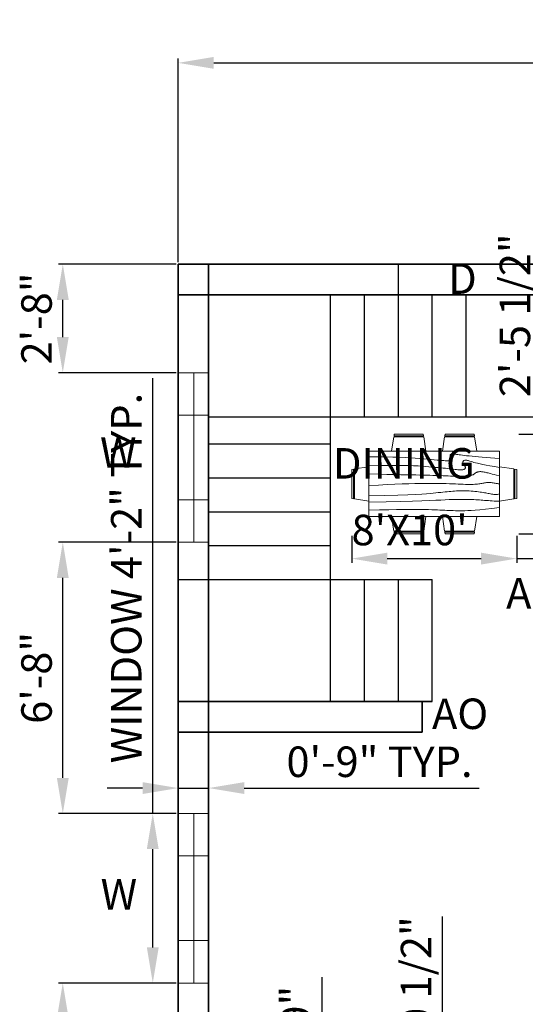
# Model space of a CAD drawing. Units: inches. Extents: x 1956 to 4770, y 1551 to 2596.
# Tile 6 of 10: x 2211 to 2361, y 2091 to 2381. Entities that reach past the tile are written whole.
import ezdxf

# ---------------------------------------------------------------- set-up
doc = ezdxf.new("R2010")
doc.units = ezdxf.units.IN
for name, color, linetype, lineweight in [('A-ANNO-DIMS', 2, 'Continuous', 18), ('A-ANNO-TEXT', 7, 'Continuous', 18), ('A-AREA-IDEN', 7, 'Continuous', 18), ('A-FLOR-STRS', 7, 'Continuous', 25), ('A-FURN', 8, 'Continuous', 18), ('A-GLAZ', 4, 'Continuous', 18), ('A-WALL', 7, 'Continuous', 35)]:
    doc.layers.add(name, color=color, linetype=linetype, lineweight=lineweight)
doc.styles.get("Standard").update_dxf_attribs({"font": 'arial.ttf'})
doc.dimstyles.new('ISO-25', dxfattribs={"dimtxt": 9, "dimasz": 10.5, "dimexe": 1.25, "dimexo": 0.625, "dimgap": 2, "dimtad": 1, "dimdec": 1, "dimlunit": 4, "dimtxsty": 'Standard', "dimcen": 2.5, "dimadec": 0, "dimazin": 0, "dimtfac": 1, "dimtdec": 1, "dimtmove": 0, "dimatfit": 3, "dimfxl": 1, "dimarcsym": 0})

# ---------------------------------------------------------------- blocks, each defined once
blk = doc.blocks.new('*D2')
at = {"layer": 'A-ANNO-DIMS', "color": 0, "lineweight": -2, "transparency": 16777216}
for p, q in [((2258.25, 2309.71), (2258.25, 2369.74)), ((2268.75, 2368.49), (2490.75, 2368.49)), ((2501.25, 2309.71), (2501.25, 2369.74))]:
    blk.add_line(p, q, dxfattribs=at)
at = {"layer": 'A-ANNO-DIMS', "color": 0, "transparency": 16777216}
for points in [[(2268.75, 2370.24), (2268.75, 2366.74), (2258.25, 2368.49)], [(2490.75, 2370.24), (2490.75, 2366.74), (2501.25, 2368.49)]]:
    blk.add_solid(points, dxfattribs=at)
at = {"layer": 'Defpoints', "color": 0, "transparency": 16777216}
for p in [(2501.25, 2368.49), (2258.25, 2309.09), (2501.25, 2309.09)]:
    blk.add_point(p, dxfattribs=at)
at = {"layer": 'A-ANNO-DIMS', "color": 0, "transparency": 16777216, "insert": (2379.75, 2375.08), "char_height": 9, "attachment_point": 5}
blk.add_mtext('20\'-3"', dxfattribs=at)
blk = doc.blocks.new('Dining Set - 36 x 72 in.')
for p, q in [((-22, 27.5), (-22.1562, 26.50042)), ((-22, 27.5), (-6, 27.5)), ((-5.8437, 26.49966), (-6, 27.5)), ((6, 27.5), (5.8438, 26.50042)), ((6, 27.5), (22, 27.5)), ((22.1563, 26.49966), (22, 27.5)), ((-22.2343, 26.00059), (-23.4847, 17.99762)), ((-22.2304, 26), (-5.7608, 26)), ((-5.8416, 26.5), (-22.1534, 26.5)), ((-4.5152, 17.99762), (-5.7655, 25.99926)), ((5.7657, 26.00059), (4.5153, 17.99762)), ((5.7696, 26), (22.2392, 26)), ((22.1584, 26.5), (5.8466, 26.5)), ((23.4848, 17.99762), (22.2345, 25.99926)), ((36, 18), (-36, 18)), ((-36, 18), (-36, -18)), ((36, -18), (36, 18)), ((-45.5, 8), (-44.5004, 8.15617)), ((-45.5, 8), (-45.5, -8)), ((-44.5, -8.15843), (-44.5, 8.15338)), ((-44.0006, 8.23428), (-35.9976, 9.48474)), ((-44, 8.23041), (-44, -8.23915)), ((44.0006, 8.23428), (35.9976, 9.48474)), ((44, 8.23041), (44, -8.23915)), ((44.5, -8.15843), (44.5, 8.15338)), ((45.5, 8), (44.5005, 8.15617)), ((45.5, 8), (45.5, -8)), ((-44.4997, -8.15631), (-45.5, -8)), ((-35.9976, -9.48476), (-43.9993, -8.2345)), ((35.9976, -9.48476), (43.9993, -8.2345)), ((44.4997, -8.15631), (45.5, -8)), ((-36, -18), (36, -18)), ((-22.2343, -26.0006), (-23.4847, -17.99762)), ((-4.5152, -17.99762), (-5.7655, -25.99928)), ((5.7657, -26.0006), (4.5153, -17.99762)), ((23.4848, -17.99762), (22.2345, -25.99928)), ((-22.2304, -26), (-5.7608, -26)), ((-22, -27.5), (-22.1562, -26.50044)), ((-5.8416, -26.5), (-22.1534, -26.5)), ((-5.8437, -26.49967), (-6, -27.5)), ((5.7696, -26), (22.2392, -26)), ((6, -27.5), (5.8438, -26.50044)), ((22.1584, -26.5), (5.8466, -26.5)), ((22.1563, -26.49967), (22, -27.5)), ((-22, -27.5), (-6, -27.5)), ((6, -27.5), (22, -27.5))]:
    blk.add_line(p, q)
for points in [[(-36, 15), (-31.1772, 14.97754), (-26.8079, 14.91406), (-22.8538, 14.81543), (-19.276, 14.6875), (-16.0362, 14.53613), (-13.0957, 14.36718), (-10.4159, 14.18652), (-7.9583, 14), (-5.6904, 13.81315), (-3.6035, 13.63021), (-1.6954, 13.45508), (0.0365, 13.29166), (1.5945, 13.14388), (2.9811, 13.01562), (4.1988, 12.9108), (5.25, 12.83333), (6.1393, 12.78613), (6.8802, 12.76823), (7.4883, 12.77767), (7.9792, 12.8125), (8.3685, 12.87077), (8.6719, 12.95052), (8.9049, 13.0498), (9.0833, 13.16666), (9.2205, 13.29899), (9.3216, 13.44401), (9.3895, 13.59879), (9.4271, 13.76041), (9.4373, 13.92594), (9.4232, 14.09245), (9.3875, 14.257), (9.3333, 14.41666), (9.2638, 14.56917), (9.1836, 14.71484), (9.0975, 14.85465), (9.0104, 14.98958), (8.9272, 15.1206), (8.8529, 15.2487), (8.7922, 15.37483), (8.75, 15.5), (8.7305, 15.62467), (8.7344, 15.74739), (8.7617, 15.86621), (8.8125, 15.97916), (8.8867, 16.08431), (8.9844, 16.17968), (9.1055, 16.26334), (9.25, 16.33333), (9.4189, 16.38802), (9.6172, 16.42708), (9.8506, 16.45052), (10.125, 16.45833), (10.4463, 16.45052), (10.8203, 16.42708), (11.2529, 16.38802), (11.75, 16.33333), (12.3184, 16.26318), (12.9694, 16.17838), (13.7151, 16.07991), (14.5677, 15.96875), (15.5395, 15.84586), (16.6426, 15.71224), (17.8893, 15.56884), (19.2917, 15.41666), (20.859, 15.25667), (22.5879, 15.08984), (24.4721, 14.91715), (26.5052, 14.73958), (28.6809, 14.5581), (30.9929, 14.3737), (33.4347, 14.18733), (36, 14)], [(-36, 10), (-28.9766, 10.14274), (-23.1725, 10.20442), (-18.4241, 10.19775), (-14.5677, 10.13541), (-11.4399, 10.03011), (-8.877, 9.89453), (-6.7154, 9.74137), (-4.7917, 9.58333), (-2.9698, 9.43082), (-1.2246, 9.28515), (0.4415, 9.14534), (2.026, 9.01041), (3.5266, 8.87939), (4.9408, 8.7513), (6.266, 8.62516), (7.5, 8.5), (8.6411, 8.37549), (9.6914, 8.2539), (10.6538, 8.13818), (11.5312, 8.03125), (12.3267, 7.93603), (13.043, 7.85547), (13.6831, 7.79248), (14.25, 7.75), (14.7471, 7.7303), (15.1797, 7.73307), (15.5537, 7.75732), (15.875, 7.80208), (16.1494, 7.86637), (16.3828, 7.94922), (16.5811, 8.04964), (16.75, 8.16666), (16.8944, 8.29915), (17.0143, 8.44531), (17.1089, 8.60319), (17.1771, 8.77083), (17.218, 8.94629), (17.2305, 9.1276), (17.2137, 9.31282), (17.1667, 9.5), (17.0895, 9.6875), (16.987, 9.875), (16.8649, 10.0625), (16.7292, 10.25), (16.5856, 10.4375), (16.4401, 10.625), (16.2985, 10.8125), (16.1667, 11), (16.05, 11.18733), (15.9518, 11.3737), (15.8752, 11.5581), (15.8229, 11.73958), (15.798, 11.91715), (15.8034, 12.08984), (15.842, 12.25667), (15.9167, 12.41666), (16.0295, 12.56836), (16.1784, 12.70833), (16.3605, 12.83268), (16.5729, 12.9375), (16.8127, 13.01888), (17.0768, 13.07291), (17.3625, 13.0957), (17.6667, 13.08333), (17.9894, 13.03312), (18.3418, 12.94726), (18.7382, 12.82918), (19.1927, 12.68229), (19.7195, 12.51001), (20.3327, 12.31575), (21.0465, 12.10294), (21.875, 11.875), (22.8357, 11.63354), (23.959, 11.37304), (25.2786, 11.08618), (26.8282, 10.76562), (28.6414, 10.40405), (30.752, 9.99414), (33.1936, 9.52856), (36, 9)], [(-36, 5.5), (-30.7157, 5.3348), (-26.069, 5.20963), (-21.9946, 5.11767), (-18.4271, 5.05208), (-15.3009, 5.00602), (-12.5508, 4.97265), (-10.1112, 4.94515), (-7.9167, 4.91666), (-5.909, 4.88167), (-4.0586, 4.83984), (-2.3429, 4.79215), (-0.7396, 4.73958), (0.7739, 4.6831), (2.22, 4.6237), (3.6213, 4.56233), (5, 4.5), (6.373, 4.43782), (7.7344, 4.3776), (9.0723, 4.32129), (10.375, 4.27083), (11.6309, 4.22819), (12.8281, 4.19531), (13.9551, 4.17415), (15, 4.16666), (15.954, 4.17448), (16.819, 4.19791), (17.6001, 4.23698), (18.3021, 4.29166), (18.9299, 4.36198), (19.4883, 4.44791), (19.9823, 4.54948), (20.4167, 4.66666), (20.7969, 4.79899), (21.1302, 4.94401), (21.4245, 5.09879), (21.6875, 5.26041), (21.9271, 5.42594), (22.1511, 5.59245), (22.3672, 5.757), (22.5834, 5.91666), (22.8065, 6.06868), (23.0404, 6.21093), (23.2879, 6.34147), (23.5521, 6.45833), (23.8358, 6.55957), (24.142, 6.64323), (24.4735, 6.70735), (24.8334, 6.75), (25.2235, 6.76969), (25.642, 6.76692), (26.0858, 6.74267), (26.5521, 6.69791), (27.0379, 6.63362), (27.5404, 6.55078), (28.0565, 6.45036), (28.5834, 6.33333), (29.1242, 6.19987), (29.7071, 6.04687), (30.3661, 5.87044), (31.1354, 5.66666), (32.0493, 5.43164), (33.142, 5.16146), (34.4475, 4.85221), (36, 4.5)], [(-36, -1), (-30.7915, -0.6591), (-26.0195, -0.38216), (-21.6519, -0.16284), (-17.6563, 0.00521), (-14.0005, 0.12833), (-10.6523, 0.21289), (-7.5796, 0.26522), (-4.75, 0.29166), (-2.134, 0.29793), (0.2878, 0.28711), (2.5317, 0.26163), (4.6146, 0.22396), (6.5529, 0.17651), (8.3633, 0.12174), (10.0623, 0.06209), (11.6667, 0), (13.1899, -0.06201), (14.6341, -0.1211), (15.9982, -0.17432), (17.2813, -0.21875), (18.4823, -0.25147), (19.6003, -0.26953), (20.6343, -0.27002), (21.5834, -0.25), (22.4481, -0.20768), (23.2357, -0.14584), (23.9549, -0.06836), (24.6146, 0.02083), (25.2235, 0.11784), (25.7904, 0.21875), (26.3241, 0.31966), (26.8334, 0.41666), (27.3265, 0.50618), (27.8099, 0.58593), (28.2894, 0.65397), (28.7709, 0.70833), (29.2601, 0.74707), (29.763, 0.76823), (30.2855, 0.76985), (30.8334, 0.75), (31.4088, 0.70784), (31.9994, 0.64713), (32.589, 0.57275), (33.1615, 0.48958), (33.7008, 0.4025), (34.1908, 0.3164), (34.6153, 0.23616), (34.9584, 0.16666), (35.2099, 0.11165), (35.3848, 0.07031), (35.504, 0.04069), (35.5886, 0.02083), (35.6594, 0.00879), (35.7377, 0.0026), (35.8442, 0.00032), (36, 0)], [(-36, -6.5), (-27.1843, -6.31267), (-20.084, -6.1263), (-14.469, -5.9419), (-10.1094, -5.76042), (-6.7752, -5.58285), (-4.2363, -5.41016), (-2.2629, -5.24333), (-0.625, -5.08334), (0.8708, -4.93099), (2.2715, -4.78646), (3.5872, -4.64974), (4.8281, -4.52084), (6.0046, -4.39974), (7.127, -4.28646), (8.2053, -4.18099), (9.25, -4.08334), (10.2705, -3.99382), (11.2734, -3.91407), (12.2647, -3.84603), (13.25, -3.79167), (14.2354, -3.75293), (15.2266, -3.73177), (16.2295, -3.73015), (17.25, -3.75), (18.2912, -3.79248), (19.3451, -3.85547), (20.4009, -3.93604), (21.4479, -4.03125), (22.4754, -4.13819), (23.4727, -4.25391), (24.4289, -4.37549), (25.3334, -4.5), (26.1785, -4.62492), (26.9694, -4.74935), (27.7145, -4.87281), (28.4219, -4.99479), (29.1, -5.11483), (29.7572, -5.23242), (30.4016, -5.34709), (31.0417, -5.45834), (31.6837, -5.56437), (32.3262, -5.65821), (32.9658, -5.73153), (33.599, -5.77604), (34.2224, -5.78345), (34.8327, -5.74545), (35.4264, -5.65373), (36, -5.5)], [(-36, -10), (-26.4022, -9.81299), (-18.4675, -9.62891), (-11.9839, -9.45069), (-6.7396, -9.28125), (-2.5226, -9.12354), (0.8789, -8.98047), (3.6769, -8.85498), (6.0833, -8.75), (8.2767, -8.66765), (10.3021, -8.60677), (12.1712, -8.56543), (13.8958, -8.54167), (15.4876, -8.53353), (16.9583, -8.53907), (18.3197, -8.55632), (19.5834, -8.58334), (20.7616, -8.61841), (21.8685, -8.66081), (22.9188, -8.71004), (23.9271, -8.76563), (24.9081, -8.82707), (25.8763, -8.89388), (26.8465, -8.96558), (27.8334, -9.04167), (28.8474, -9.12118), (29.8828, -9.20117), (30.93, -9.27824), (31.9792, -9.34896), (33.0205, -9.40991), (34.0443, -9.45768), (35.0407, -9.48885), (36, -9.5)], [(-36, -14.5), (-30.0881, -14.33513), (-25.0332, -14.21224), (-20.7312, -14.12647), (-17.0781, -14.07292), (-13.97, -14.04671), (-11.3027, -14.04297), (-8.9724, -14.05681), (-6.875, -14.08334), (-4.9224, -14.11833), (-3.0905, -14.16016), (-1.3709, -14.20785), (0.2448, -14.26042), (1.7647, -14.3169), (3.1973, -14.3763), (4.5507, -14.43767), (5.8333, -14.5), (7.0554, -14.5621), (8.235, -14.62175), (9.3922, -14.67652), (10.5469, -14.72396), (11.7192, -14.76164), (12.929, -14.78711), (14.1965, -14.79794), (15.5417, -14.79167), (16.9933, -14.76424), (18.6152, -14.70508), (20.4804, -14.60197), (22.6615, -14.44271), (25.2312, -14.21509), (28.2624, -13.9069), (31.8277, -13.50594), (36, -13)]]:
    blk.add_lwpolyline(points)
blk = doc.blocks.new('WIN-50IN-WALL9')
for p, q in [((0, 50), (9, 50)), ((4.6, 50), (4.6, 0)), ((0, 37.5), (9, 37.5)), ((9, 12.5), (0, 12.5)), ((9, 0), (1, 0)), ((0, 0), (9, 0))]:
    blk.add_line(p, q)
blk = doc.blocks.new('*D27')
at = {"layer": 'A-ANNO-DIMS', "color": 0, "lineweight": -2, "transparency": 16777216}
for p, q in [((2250.75, 2147.09), (2250.75, 2275.47)), ((2257.63, 2147.09), (2249.5, 2147.09)), ((2250.75, 2107.59), (2250.75, 2136.59)), ((2257.63, 2097.09), (2249.5, 2097.09))]:
    blk.add_line(p, q, dxfattribs=at)
at = {"layer": 'A-ANNO-DIMS', "color": 0, "transparency": 16777216}
for points in [[(2249, 2136.59), (2252.5, 2136.59), (2250.75, 2147.09)], [(2249, 2107.59), (2252.5, 2107.59), (2250.75, 2097.09)]]:
    blk.add_solid(points, dxfattribs=at)
at = {"layer": 'Defpoints', "color": 0, "transparency": 16777216}
for p in [(2250.75, 2147.09), (2258.25, 2147.09), (2258.25, 2097.09)]:
    blk.add_point(p, dxfattribs=at)
at = {"layer": 'A-ANNO-DIMS', "color": 0, "transparency": 16777216, "insert": (2244.1, 2216.53), "char_height": 9, "attachment_point": 5, "rotation": 90}
blk.add_mtext('WINDOW 4\'-2" TYP.', dxfattribs=at)
blk = doc.blocks.new('*D28')
at = {"layer": 'A-ANNO-DIMS', "color": 0, "lineweight": -2, "transparency": 16777216}
for p, q in [((2258.25, 2147.71), (2258.25, 2155.84)), ((2267.25, 2147.71), (2267.25, 2155.84)), ((2247.75, 2154.59), (2237.25, 2154.59)), ((2258.25, 2154.59), (2267.25, 2154.59)), ((2277.75, 2154.59), (2347.11, 2154.59))]:
    blk.add_line(p, q, dxfattribs=at)
at = {"layer": 'A-ANNO-DIMS', "color": 0, "transparency": 16777216}
for points in [[(2247.75, 2156.34), (2247.75, 2152.84), (2258.25, 2154.59)], [(2277.75, 2156.34), (2277.75, 2152.84), (2267.25, 2154.59)]]:
    blk.add_solid(points, dxfattribs=at)
at = {"layer": 'Defpoints', "color": 0, "transparency": 16777216}
for p in [(2267.25, 2154.59), (2258.25, 2147.09), (2267.25, 2147.09)]:
    blk.add_point(p, dxfattribs=at)
at = {"layer": 'A-ANNO-DIMS', "color": 0, "transparency": 16777216, "insert": (2317.68, 2161.18), "char_height": 9, "attachment_point": 5}
blk.add_mtext('0\'-9" TYP.', dxfattribs=at)
blk = doc.blocks.new('*D32')
at = {"layer": 'A-ANNO-DIMS', "color": 0, "lineweight": -2, "transparency": 16777216}
for p, q in [((2336.28, 2051.19), (2336.28, 2116.73)), ((2331.39, 2040.69), (2337.53, 2040.69)), ((2336.28, 2018.23), (2336.28, 2040.69)), ((2331.39, 2018.23), (2337.53, 2018.23)), ((2336.28, 2007.73), (2336.28, 1997.23))]:
    blk.add_line(p, q, dxfattribs=at)
at = {"layer": 'A-ANNO-DIMS', "color": 0, "transparency": 16777216}
for points in [[(2334.53, 2051.19), (2338.03, 2051.19), (2336.28, 2040.69)], [(2334.53, 2007.73), (2338.03, 2007.73), (2336.28, 2018.23)]]:
    blk.add_solid(points, dxfattribs=at)
at = {"layer": 'Defpoints', "color": 0, "transparency": 16777216}
for p in [(2330.76, 2040.69), (2336.28, 2040.69), (2330.76, 2018.23)]:
    blk.add_point(p, dxfattribs=at)
at = {"layer": 'A-ANNO-DIMS', "color": 0, "transparency": 16777216, "insert": (2329.63, 2089.21), "char_height": 9, "attachment_point": 5, "rotation": 90}
blk.add_mtext('1\'-10 1/2"', dxfattribs=at)
blk = doc.blocks.new('*D35')
at = {"layer": 'A-ANNO-DIMS', "color": 0, "lineweight": -2, "transparency": 16777216}
for p, q in [((2300.74, 2022.72), (2300.74, 2098.83)), ((2294.63, 2022.72), (2301.99, 2022.72)), ((2300.74, 1988.27), (2300.74, 2012.22)), ((2294.63, 1977.77), (2301.99, 1977.77))]:
    blk.add_line(p, q, dxfattribs=at)
at = {"layer": 'A-ANNO-DIMS', "color": 0, "transparency": 16777216}
for points in [[(2298.99, 2012.22), (2302.49, 2012.22), (2300.74, 2022.72)], [(2298.99, 1988.27), (2302.49, 1988.27), (2300.74, 1977.77)]]:
    blk.add_solid(points, dxfattribs=at)
at = {"layer": 'Defpoints', "color": 0, "transparency": 16777216}
for p in [(2294, 2022.72), (2300.74, 2022.72), (2294, 1977.77)]:
    blk.add_point(p, dxfattribs=at)
at = {"layer": 'A-ANNO-DIMS', "color": 0, "transparency": 16777216, "insert": (2294.08, 2066.02), "char_height": 9, "attachment_point": 5, "rotation": 90}
blk.add_mtext('SOFA 3\'-9"', dxfattribs=at)
blk = doc.blocks.new('*D51')
at = {"layer": 'A-ANNO-DIMS', "color": 0, "lineweight": -2, "transparency": 16777216}
for p, q in [((2309.47, 2228.95), (2309.47, 2221.02)), ((2358.16, 2228.95), (2358.16, 2221.02)), ((2319.97, 2222.27), (2347.66, 2222.27)), ((2358.16, 2222.27), (2492.55, 2222.27))]:
    blk.add_line(p, q, dxfattribs=at)
at = {"layer": 'A-ANNO-DIMS', "color": 0, "transparency": 16777216}
for points in [[(2319.97, 2224.02), (2319.97, 2220.52), (2309.47, 2222.27)], [(2347.66, 2224.02), (2347.66, 2220.52), (2358.16, 2222.27)]]:
    blk.add_solid(points, dxfattribs=at)
at = {"layer": 'Defpoints', "color": 0, "transparency": 16777216}
for p in [(2309.47, 2229.57), (2358.16, 2229.57), (2358.16, 2222.27)]:
    blk.add_point(p, dxfattribs=at)
at = {"layer": 'A-ANNO-DIMS', "color": 0, "transparency": 16777216, "insert": (2430.61, 2228.92), "char_height": 9, "attachment_point": 5}
blk.add_mtext('DINING SET 4\'-0 1/2"', dxfattribs=at)
blk = doc.blocks.new('*D52')
at = {"layer": 'A-ANNO-DIMS', "color": 0, "lineweight": -2, "transparency": 16777216}
for p, q in [((2365.47, 2259), (2365.47, 2318.55)), ((2358.79, 2259), (2366.72, 2259)), ((2365.47, 2240.07), (2365.47, 2248.5)), ((2358.79, 2229.57), (2366.72, 2229.57))]:
    blk.add_line(p, q, dxfattribs=at)
at = {"layer": 'A-ANNO-DIMS', "color": 0, "transparency": 16777216}
for points in [[(2363.72, 2248.5), (2367.22, 2248.5), (2365.47, 2259)], [(2363.72, 2240.07), (2367.22, 2240.07), (2365.47, 2229.57)]]:
    blk.add_solid(points, dxfattribs=at)
at = {"layer": 'Defpoints', "color": 0, "transparency": 16777216}
for p in [(2358.16, 2259), (2365.47, 2259), (2358.16, 2229.57)]:
    blk.add_point(p, dxfattribs=at)
at = {"layer": 'A-ANNO-DIMS', "color": 0, "transparency": 16777216, "insert": (2358.81, 2294.03), "char_height": 9, "attachment_point": 5, "rotation": 90}
blk.add_mtext('2\'-5 1/2"', dxfattribs=at)
blk = doc.blocks.new('*D66')
at = {"layer": 'A-ANNO-DIMS', "color": 0, "lineweight": -2, "transparency": 16777216}
for p, q in [((2257.63, 2097.09), (2222.95, 2097.09)), ((2224.2, 2002.59), (2224.2, 2086.59)), ((2257.63, 1992.09), (2222.95, 1992.09))]:
    blk.add_line(p, q, dxfattribs=at)
at = {"layer": 'A-ANNO-DIMS', "color": 0, "transparency": 16777216}
for points in [[(2222.45, 2086.59), (2225.95, 2086.59), (2224.2, 2097.09)], [(2222.45, 2002.59), (2225.95, 2002.59), (2224.2, 1992.09)]]:
    blk.add_solid(points, dxfattribs=at)
at = {"layer": 'Defpoints', "color": 0, "transparency": 16777216}
for p in [(2224.2, 2097.09), (2258.25, 2097.09), (2258.25, 1992.09)]:
    blk.add_point(p, dxfattribs=at)
at = {"layer": 'A-ANNO-DIMS', "color": 0, "transparency": 16777216, "insert": (2217.61, 2044.59), "char_height": 9, "attachment_point": 5, "rotation": 90}
blk.add_mtext('8\'-9"', dxfattribs=at)
blk = doc.blocks.new('*D67')
at = {"layer": 'A-ANNO-DIMS', "color": 0, "lineweight": -2, "transparency": 16777216}
for p, q in [((2257.63, 2227.09), (2222.95, 2227.09)), ((2224.2, 2157.59), (2224.2, 2216.59)), ((2257.63, 2147.09), (2222.95, 2147.09))]:
    blk.add_line(p, q, dxfattribs=at)
at = {"layer": 'A-ANNO-DIMS', "color": 0, "transparency": 16777216}
for points in [[(2222.45, 2216.59), (2225.95, 2216.59), (2224.2, 2227.09)], [(2222.45, 2157.59), (2225.95, 2157.59), (2224.2, 2147.09)]]:
    blk.add_solid(points, dxfattribs=at)
at = {"layer": 'Defpoints', "color": 0, "transparency": 16777216}
for p in [(2224.2, 2227.09), (2258.25, 2227.09), (2258.25, 2147.09)]:
    blk.add_point(p, dxfattribs=at)
at = {"layer": 'A-ANNO-DIMS', "color": 0, "transparency": 16777216, "insert": (2217.61, 2187.09), "char_height": 9, "attachment_point": 5, "rotation": 90}
blk.add_mtext('6\'-8"', dxfattribs=at)
blk = doc.blocks.new('*D68')
at = {"layer": 'A-ANNO-DIMS', "color": 0, "lineweight": -2, "transparency": 16777216}
for p, q in [((2257.63, 2309.09), (2222.95, 2309.09)), ((2224.2, 2287.59), (2224.2, 2298.59)), ((2257.63, 2277.09), (2222.95, 2277.09))]:
    blk.add_line(p, q, dxfattribs=at)
at = {"layer": 'A-ANNO-DIMS', "color": 0, "transparency": 16777216}
for points in [[(2222.45, 2298.59), (2225.95, 2298.59), (2224.2, 2309.09)], [(2222.45, 2287.59), (2225.95, 2287.59), (2224.2, 2277.09)]]:
    blk.add_solid(points, dxfattribs=at)
at = {"layer": 'Defpoints', "color": 0, "transparency": 16777216}
for p in [(2224.2, 2309.09), (2258.25, 2309.09), (2258.25, 2277.09)]:
    blk.add_point(p, dxfattribs=at)
at = {"layer": 'A-ANNO-DIMS', "color": 0, "transparency": 16777216, "insert": (2217.61, 2293.09), "char_height": 9, "attachment_point": 5, "rotation": 90}
blk.add_mtext('2\'-8"', dxfattribs=at)

msp = doc.modelspace()

# ---------------------------------------------------------------- linework, layer by layer
at = {"layer": 'A-FLOR-STRS'}
for p, q in [((2323.25, 2264.09), (2323.25, 2309.09)), ((2303.25, 2180.09), (2303.25, 2300.09)), ((2313.25, 2264.09), (2313.25, 2300.09)), ((2333.25, 2264.09), (2333.25, 2300.09)), ((2343.25, 2264.09), (2343.25, 2300.09)), ((2267.25, 2264.09), (2303.25, 2264.09)), ((2303.25, 2264.09), (2363.25, 2264.09)), ((2267.25, 2256.09), (2303.25, 2256.09)), ((2267.25, 2246.09), (2303.25, 2246.09)), ((2267.25, 2236.09), (2303.25, 2236.09)), ((2267.25, 2226.09), (2303.25, 2226.09)), ((2258.25, 2216.09), (2333.25, 2216.09)), ((2313.25, 2180.09), (2313.25, 2216.09)), ((2323.25, 2180.09), (2323.25, 2216.09)), ((2333.25, 2180.09), (2333.25, 2216.09))]:
    msp.add_line(p, q, dxfattribs=at)
at = {"layer": 'A-GLAZ'}
for p, q in [((2258.25, 2277.09), (2267.25, 2277.09)), ((2258.25, 2227.09), (2267.25, 2227.09)), ((2258.25, 2147.09), (2267.25, 2147.09))]:
    msp.add_line(p, q, dxfattribs=at)
at = {"layer": 'A-WALL'}
for p, q in [((2258.25, 2309.09), (2501.25, 2309.09)), ((2258.25, 1757.09), (2258.25, 2309.09)), ((2267.25, 1910.09), (2267.25, 2309.09)), ((2258.25, 2300.09), (2492.25, 2300.09)), ((2258.25, 2180.09), (2333.25, 2180.09)), ((2330.25, 2171.09), (2330.25, 2180.09)), ((2258.25, 2171.09), (2330.25, 2171.09))]:
    msp.add_line(p, q, dxfattribs=at)

# ---------------------------------------------------------------- block references
at = {"layer": 'A-FURN', "xscale": 0.5351030771477641, "yscale": 0.5351030771477641, "zscale": 0.5351030771477641}
msp.add_blockref('Dining Set - 36 x 72 in.', (2333.81, 2244.29), dxfattribs=at)
at = {"layer": 'A-GLAZ'}
for p in [(2258.25, 2227.09), (2258.25, 2097.09)]:
    msp.add_blockref('WIN-50IN-WALL9', p, dxfattribs=at)

# ---------------------------------------------------------------- texts
at = {"layer": 'A-ANNO-TEXT'}
for s, p in [('D', (2337.93, 2300.34)), ('         W ', (2210.43, 2249.04)), ('        AO', (2333.05, 2207.53)), ('        AO', (2311.17, 2172)), ('         W ', (2210.61, 2118.76))]:
    msp.add_text(s, height=9, dxfattribs=at).set_placement(p)
at = {"layer": 'A-AREA-IDEN'}
for s, p in [('DINING', (2303.91, 2245.86)), ("  8'X10'", (2303.91, 2226.2))]:
    msp.add_text(s, height=9, dxfattribs=at).set_placement(p)

# ---------------------------------------------------------------- dimensions: what is measured, and where the dimension line sits
at = {"layer": 'A-ANNO-DIMS'}
dim = msp.add_linear_dim(base=(2501.25, 2368.49), p1=(2258.25, 2309.09), p2=(2501.25, 2309.09), dimstyle='ISO-25', override={"dimclrd": 0, "dimclre": 0, "dimclrt": 0}, dxfattribs=at)
dim.commit()
dim.dimension.update_dxf_attribs({"geometry": '*D2', "text_midpoint": (2379.75, 2375.08)})
for base, p1, p2, picture, middle in [((2365.47, 2259), (2358.16, 2229.57), (2358.16, 2259), '*D52', (2358.81, 2294.03)), ((2224.2, 2309.09), (2258.25, 2277.09), (2258.25, 2309.09), '*D68', (2217.61, 2293.09)), ((2224.2, 2227.09), (2258.25, 2147.09), (2258.25, 2227.09), '*D67', (2217.61, 2187.09)), ((2336.28, 2040.69), (2330.76, 2018.23), (2330.76, 2040.69), '*D32', (2329.63, 2089.21)), ((2224.2, 2097.09), (2258.25, 1992.09), (2258.25, 2097.09), '*D66', (2217.61, 2044.59))]:
    dim = msp.add_linear_dim(base=base, p1=p1, p2=p2, angle=90, dimstyle='ISO-25', override={"dimdec": 1, "dimlfac": 1, "dimrnd": 0, "dimzin": 1, "dimdsep": 46, "dimlunit": 4, "dimfrac": 2}, dxfattribs=at)
    dim.commit()
    dim.dimension.update_dxf_attribs({"geometry": picture, "text_midpoint": middle})
for base, p1, p2, text, picture, middle in [((2250.75, 2147.09), (2258.25, 2097.09), (2258.25, 2147.09), 'WINDOW <> TYP.', '*D27', (2244.1, 2216.53)), ((2300.7428, 2022.7213), (2294.0005, 1977.7726), (2294.0005, 2022.7213), 'SOFA <>', '*D35', (2294.0832, 2066.0245))]:
    dim = msp.add_linear_dim(base=base, p1=p1, p2=p2, angle=90, text=text, dimstyle='ISO-25', override={"dimdec": 1, "dimlfac": 1, "dimrnd": 0, "dimzin": 1, "dimdsep": 46, "dimlunit": 4, "dimfrac": 2}, dxfattribs=at)
    dim.commit()
    dim.dimension.update_dxf_attribs({"geometry": picture, "text_midpoint": middle})
for base, p1, p2, text, picture, middle in [((2358.16, 2222.27), (2309.47, 2229.57), (2358.16, 2229.57), 'DINING SET <>', '*D51', (2430.61, 2228.92)), ((2267.25, 2154.59), (2258.25, 2147.09), (2267.25, 2147.09), '<> TYP.', '*D28', (2317.68, 2161.18))]:
    dim = msp.add_linear_dim(base=base, p1=p1, p2=p2, text=text, dimstyle='ISO-25', override={"dimdec": 1, "dimlfac": 1, "dimrnd": 0, "dimzin": 1, "dimdsep": 46, "dimlunit": 4, "dimfrac": 2}, dxfattribs=at)
    dim.commit()
    dim.dimension.update_dxf_attribs({"geometry": picture, "text_midpoint": middle})

doc.saveas('drawing.dxf')
